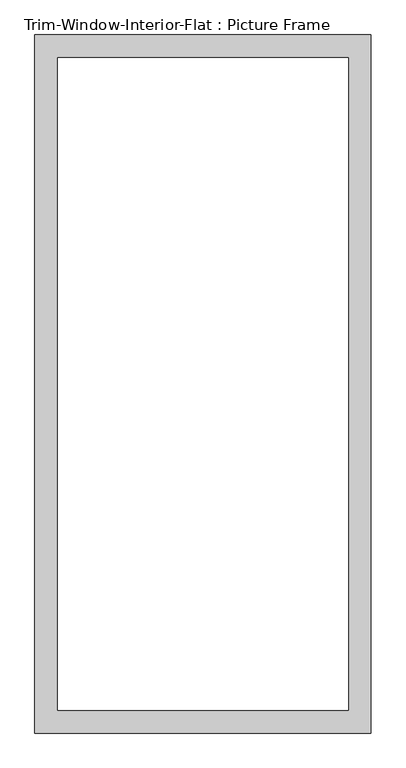
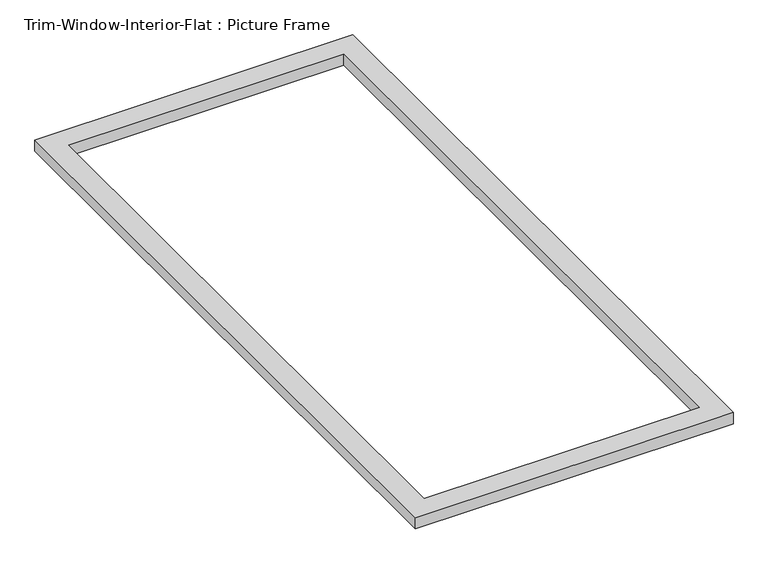
"""IFC4 building model written with IfcOpenShell, lengths in millimetres: proxy geometry, Trim-Window-Interior-Flat : Picture Frame."""

from ifc_helpers import new_model, si_unit, origin, origin_with_axes, place, context, project, spatial, polyline, outline, extrude, source, transform, mapped, element, save


def trim_window_interior_flat_picture_frame_129e3d92(model_context):
    return source(origin(), model_context, "Body", "SweptSolid", [
        extrude(outline(polyline([(425.45, 44.45), (425.45, -1720.85), (-425.45, -1720.85), (-425.45, 44.45), (425.45, 44.45)]), holes=[polyline([(368.3, -12.7), (-368.3, -12.7), (-368.3, -1663.7), (368.3, -1663.7), (368.3, -12.7)])]), origin_with_axes(), (0.0, 0.0, 1.0), 31.75),
    ])


if __name__ == "__main__":
    model = new_model("IFC4")
    model_context = context("Model", 3, world=origin())
    ifc_project = project(units=[si_unit("LENGTHUNIT", "METRE", prefix="MILLI")], contexts=[model_context])
    site = spatial("IfcSite", under=ifc_project)
    building = spatial("IfcBuilding", under=site)
    placement = place(None, origin())
    trim_window_interior_flat_picture_frame_shape = trim_window_interior_flat_picture_frame_129e3d92(model_context)
    element("IfcBuildingElementProxy", 1, Name="Trim-Window-Interior-Flat : Picture Frame", ObjectType="Trim-Window-Interior-Flat : Picture Frame", at=placement, inside=building, context=model_context, shape_type="MappedRepresentation", body=[
        mapped(trim_window_interior_flat_picture_frame_shape, transform((0.0, 0.0, 0.0), x_axis=(1.0, 0.0, 0.0), y_axis=(0.0, 1.0, 0.0), z_axis=(0.0, 0.0, 1.0))),
    ])
    save(model, "model.ifc")

# Revit data of these elements
# Type "Trim-Window-Interior-Flat : Picture Frame"
#   Trim Thickness_Picture Frame = 0' - 1 1/4"
#   Trim Width = 0' - 2 1/4"
#   Trim Thickness_with Sill = 0' - 0 3/4"
#   Sill Thickness = 0' - 1 1/4"
#   Opening Width [instance default] = 2' - 0"
#   Opening Height [instance default] = 3' - 0"
#   Default Elevation = 4' - 0"
#   Sill = no
#   Picture Frame = yes
#   Trim Material [instance default] = none
# Element 1 (IfcBuildingElementProxy, "Trim-Window-Interior-Flat : Picture Frame")
#   Opening Width = 2' - 6"
#   Opening Height = 5' - 6"
#   Trim Material = Wood - Stained
#   Materials on its faces: "Wood - Stained"
# Materials
#   "Wood - Stained": class "Wood", colour RGB 224 178 126, transparency 0, Cost = 0
